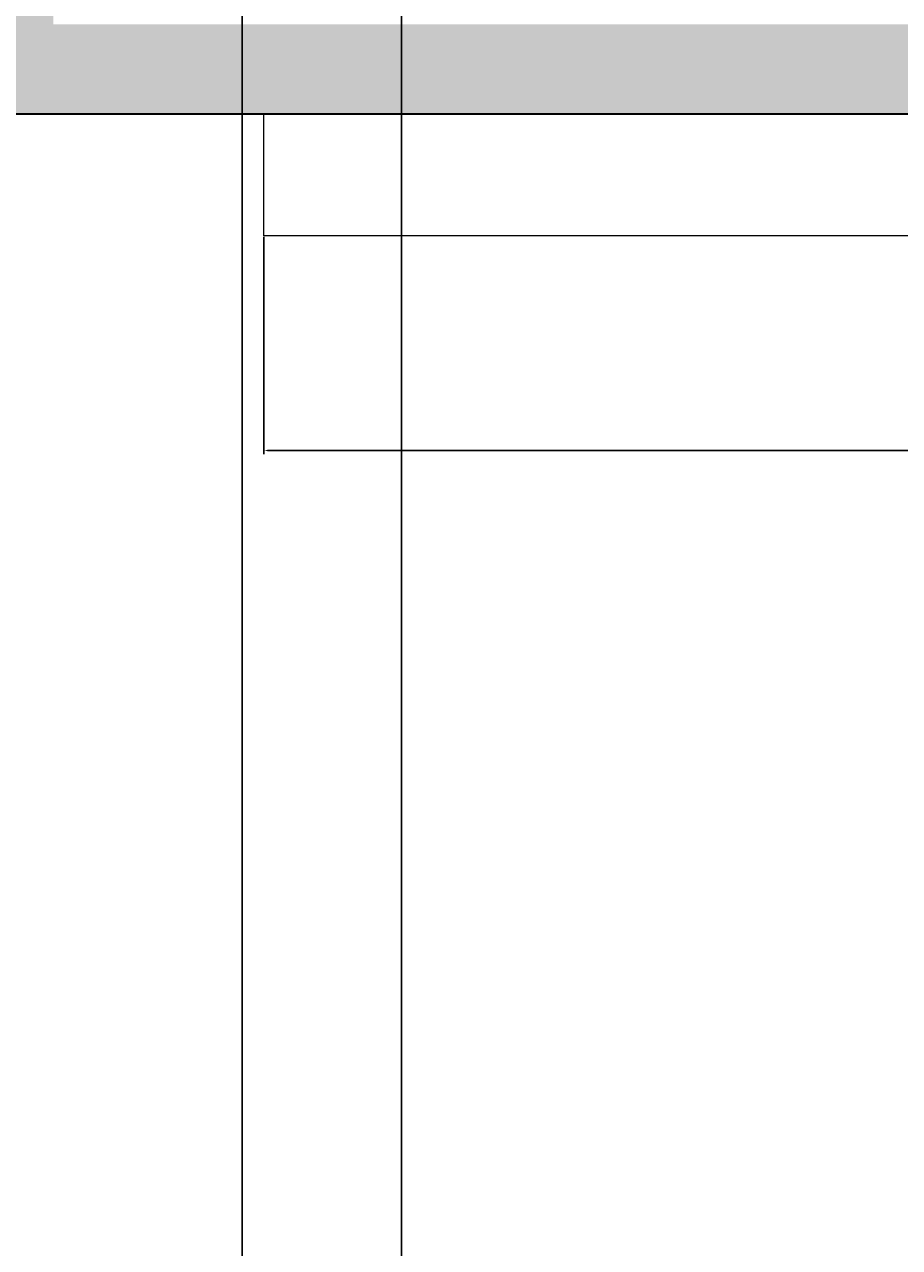
# Model space of a CAD drawing. Units: inches. Extents: x 1998 to 2588, y 1139 to 1977.
# Tile 128 of 134: x 2397 to 2441, y 1698 to 1760. Entities that reach past the tile are written whole.
import ezdxf

# ---------------------------------------------------------------- set-up
doc = ezdxf.new("R2010")
doc.units = ezdxf.units.IN
for name, color, linetype, lineweight in [('A-ANNO-DIMS', 2, 'Continuous', 18), ('A-WALL-PATT', 252, 'Continuous', 13), ('FUR', 21, 'Continuous', 18), ('WALL', 200, 'Continuous', 35)]:
    doc.layers.add(name, color=color, linetype=linetype, lineweight=lineweight)
doc.styles.get("Standard").update_dxf_attribs({"font": 'arial.ttf'})
doc.dimstyles.get("Standard").update_dxf_attribs({"dimtxt": 0.18, "dimasz": 0.18, "dimexe": 0.18, "dimexo": 0.0625, "dimgap": 0.09, "dimtad": 0, "dimtih": 1, "dimtoh": 1, "dimdec": 4, "dimzin": 0, "dimdsep": 46, "dimtxsty": 'Standard', "dimcen": 0.09, "dimadec": 0, "dimazin": 0, "dimtfac": 1, "dimtdec": 4, "dimtofl": 0, "dimtmove": 0, "dimatfit": 3, "dimfxl": 1, "dimtolj": 1, "dimtzin": 0, "dimarcsym": 0})

# ---------------------------------------------------------------- blocks, each defined once
blk = doc.blocks.new('CONSOLE-WALL')
blk.add_lwpolyline([(0, 6.123), (71.98, 6.123), (71.98, 0), (0, 0)], close=True)
blk = doc.blocks.new('*D17')
at = {"layer": 'A-ANNO-DIMS', "color": 0, "lineweight": -2, "transparency": 16777216}
for p, q in [((2409.062, 1749.046), (2409.062, 1738.132)), ((2481.042, 1749.046), (2481.042, 1738.132)), ((2409.242, 1738.312), (2443.875, 1738.312)), ((2480.862, 1738.312), (2446.228, 1738.312))]:
    blk.add_line(p, q, dxfattribs=at)
at = {"layer": 'A-ANNO-DIMS', "color": 0, "transparency": 16777216}
for points in [[(2409.242, 1738.342), (2409.242, 1738.282), (2409.062, 1738.312)], [(2480.862, 1738.342), (2480.862, 1738.282), (2481.042, 1738.312)]]:
    blk.add_solid(points, dxfattribs=at)
at = {"layer": 'Defpoints', "color": 0, "transparency": 16777216}
for p in [(2409.062, 1749.109), (2481.042, 1749.109), (2481.042, 1738.312)]:
    blk.add_point(p, dxfattribs=at)
at = {"layer": 'A-ANNO-DIMS', "color": 0, "transparency": 16777216, "insert": (2445.052, 1738.312), "char_height": 0.18, "attachment_point": 5}
blk.add_mtext('\\A1;CONSOLE 72 TYP.', dxfattribs=at)
blk = doc.blocks.new('*D24')
at = {"layer": 'A-ANNO-DIMS', "color": 0, "lineweight": -2, "transparency": 16777216}
for p, q in [((2398.535, 1911.232), (2588.309, 1911.232)), ((2588.129, 1911.052), (2588.129, 1570.164)), ((2588.129, 1228.912), (2588.129, 1569.8)), ((2527.535, 1228.732), (2588.309, 1228.732))]:
    blk.add_line(p, q, dxfattribs=at)
at = {"layer": 'A-ANNO-DIMS', "color": 0, "transparency": 16777216}
for points in [[(2588.099, 1911.052), (2588.159, 1911.052), (2588.129, 1911.232)], [(2588.099, 1228.912), (2588.159, 1228.912), (2588.129, 1228.732)]]:
    blk.add_solid(points, dxfattribs=at)
at = {"layer": 'Defpoints', "color": 0, "transparency": 16777216}
for p in [(2398.473, 1911.232), (2588.129, 1911.232), (2527.473, 1228.732)]:
    blk.add_point(p, dxfattribs=at)
at = {"layer": 'A-ANNO-DIMS', "color": 0, "transparency": 16777216, "insert": (2588.129, 1569.982), "char_height": 0.18, "attachment_point": 5}
blk.add_mtext('\\A1;682.5', dxfattribs=at)
blk = doc.blocks.new('*D32')
at = {"layer": 'A-ANNO-DIMS', "color": 0, "lineweight": -2, "transparency": 16777216}
for p, q in [((2407.973, 1636.795), (2407.973, 1977.362)), ((2415.973, 1636.795), (2415.973, 1977.362)), ((2408.153, 1977.182), (2411.824, 1977.182)), ((2415.793, 1977.182), (2412.122, 1977.182))]:
    blk.add_line(p, q, dxfattribs=at)
at = {"layer": 'A-ANNO-DIMS', "color": 0, "transparency": 16777216}
for points in [[(2408.153, 1977.212), (2408.153, 1977.152), (2407.973, 1977.182)], [(2415.793, 1977.212), (2415.793, 1977.152), (2415.973, 1977.182)]]:
    blk.add_solid(points, dxfattribs=at)
at = {"layer": 'Defpoints', "color": 0, "transparency": 16777216}
for p in [(2415.973, 1977.182), (2407.973, 1636.732), (2415.973, 1636.732)]:
    blk.add_point(p, dxfattribs=at)
at = {"layer": 'A-ANNO-DIMS', "color": 0, "transparency": 16777216, "insert": (2411.973, 1977.182), "char_height": 0.18, "attachment_point": 5}
blk.add_mtext('\\A1;8', dxfattribs=at)

msp = doc.modelspace()

# ---------------------------------------------------------------- hatches: boundary and pattern name
at = {"layer": 'A-WALL-PATT'}
h = msp.add_hatch(color=256, dxfattribs=at)
h.dxf.hatch_style = 1
h.paths.add_polyline_path([(2227.4729, 1911.2324), (2222.9729, 1911.2324), (2222.9729, 1888.7324), (2227.4729, 1888.7324)])
h.paths.add_polyline_path([(2236.4493, 1870.3636), (2236.4493, 1875.2324), (2234.4125, 1875.2324), (2234.4125, 1868.3278), (2227.4729, 1868.3278), (2227.4729, 1866.2324), (2236.4493, 1866.2324)])
h.paths.add_polyline_path([(2330.0332, 1875.2324), (2263.9907, 1875.2324), (2263.9907, 1866.2324), (2330.0332, 1866.2324)])
h.paths.add_polyline_path([(2345.9729, 1906.7324), (2393.9729, 1906.7324), (2393.9729, 1882.7324), (2345.9729, 1882.7324), (2345.9729, 1878.2324), (2393.9729, 1878.2324), (2398.4729, 1878.2324), (2398.4729, 1882.7324), (2398.4729, 1911.2324), (2345.9729, 1911.2324), (2341.4729, 1911.2324), (2341.4729, 1866.2324), (2341.4729, 1790.0412), (2345.9729, 1790.0412), (2345.9729, 1875.2324)])
h.paths.add_polyline_path([(2398.4729, 1878.2324), (2393.9729, 1878.2324), (2393.9729, 1798.2324), (2393.9729, 1793.7324), (2398.4729, 1793.7324)], flags=17)
h.paths.add_polyline_path([(2393.9729, 1798.2324), (2375.7311, 1798.2324, -0.005968), (2375.7384, 1797.6146), (2375.7384, 1793.7324), (2393.9729, 1793.7324)], flags=17)
h.paths.add_polyline_path([(2349.8569, 1797.6146), (2349.8569, 1798.2324), (2345.9729, 1798.2324), (2345.9729, 1793.7324), (2349.8569, 1793.7324)], flags=17)
h.paths.add_polyline_path([(2398.4729, 1793.7324), (2393.9729, 1793.7324), (2393.9729, 1790.0412), (2398.4729, 1790.0412)], flags=17)
h.paths.add_polyline_path([(2527.4729, 1882.7324), (2507.8006, 1882.7324), (2507.8006, 1878.2324), (2518.4729, 1878.2324), (2518.4729, 1759.7324), (2510.9729, 1759.7324), (2510.9729, 1755.2324), (2527.4729, 1755.2324)])
h.paths.add_polyline_path([(2487.396, 1882.7324), (2398.4729, 1882.7324), (2398.4729, 1878.2324), (2487.396, 1878.2324)])
h.paths.add_polyline_path([(2490.5682, 1759.7324), (2345.9729, 1759.7324), (2345.9729, 1755.2324), (2490.5682, 1755.2324)])
h.paths.add_polyline_path([(2398.4729, 1760.5844), (2398.3914, 1760.5844), (2393.9729, 1760.5844), (2393.9729, 1759.7324), (2398.4729, 1759.7324)])
h.paths.add_polyline_path([(2334.5332, 1759.7324), (2234.4125, 1759.7324), (2234.4125, 1755.2324), (2334.5332, 1755.2324)])
h.paths.add_polyline_path([(2345.9729, 1760.5844), (2341.5543, 1760.5844), (2341.4729, 1760.5844), (2341.4729, 1759.7324), (2345.9729, 1759.7324)])
h.paths.add_polyline_path([(2222.9729, 1759.7324), (2221.7204, 1759.7324), (2221.7204, 1755.2324), (2222.9729, 1755.2324)])
h.paths.add_polyline_path([(2061.4729, 1702.7324), (2059.4729, 1702.7324), (2059.4729, 1584.2324), (2061.4729, 1584.2324)])
h.paths.add_polyline_path([(2061.4729, 1584.2324), (2059.4729, 1584.2324), (2059.4729, 1470.2324), (2061.4729, 1470.2324)])
h.paths.add_polyline_path([(2510.9729, 1469.2927), (2501.9729, 1469.2927), (2501.9729, 1369.172), (2510.9729, 1369.172)])
h.paths.add_polyline_path([(2227.4729, 1369.7324), (2227.4729, 1417.7324), (2221.4126, 1417.7324), (2221.4126, 1413.2324), (2222.9729, 1413.2324), (2222.9729, 1293.2324), (2222.9729, 1285.137), (2227.4729, 1285.137)])

# ---------------------------------------------------------------- linework, layer by layer
at = {"layer": 'WALL'}
for q in [(2527.4729, 1755.2324), (2501.9729, 1755.2324)]:
    msp.add_line((2345.9729, 1755.2324), q, dxfattribs=at)

# ---------------------------------------------------------------- block references
at = {"layer": 'FUR'}
msp.add_blockref('CONSOLE-WALL', (2409.062, 1749.109), dxfattribs=at)

# ---------------------------------------------------------------- dimensions: what is measured, and where the dimension line sits
at = {"layer": 'A-ANNO-DIMS'}
dim = msp.add_linear_dim(base=(2415.9729, 1977.1824), p1=(2407.9729, 1636.7324), p2=(2415.9729, 1636.7324), dimstyle='Standard', override={"dimdec": 0, "dimlfac": 1, "dimrnd": 0, "dimzin": 0, "dimdsep": 46, "dimlunit": 2}, dxfattribs=at)
dim.commit()
dim.dimension.update_dxf_attribs({"geometry": '*D32', "text_midpoint": (2411.9729, 1977.1824)})
dim = msp.add_linear_dim(base=(2588.1286, 1911.2324), p1=(2527.4729, 1228.7324), p2=(2398.4729, 1911.2324), angle=90, dimstyle='Standard', override={"dimdec": 1, "dimlfac": 1, "dimrnd": 0, "dimzin": 0, "dimdsep": 46, "dimlunit": 2}, dxfattribs=at)
dim.commit()
dim.dimension.update_dxf_attribs({"geometry": '*D24', "text_midpoint": (2588.1286, 1569.9824)})
dim = msp.add_linear_dim(base=(2481.0415, 1738.312), p1=(2409.0618, 1749.1089), p2=(2481.0415, 1749.1089), text='CONSOLE <> TYP.', dimstyle='Standard', override={"dimdec": 0, "dimlfac": 1, "dimrnd": 0, "dimzin": 0, "dimdsep": 46, "dimlunit": 2}, dxfattribs=at)
dim.commit()
dim.dimension.update_dxf_attribs({"geometry": '*D17', "text_midpoint": (2445.0517, 1738.312)})

doc.saveas('drawing.dxf')
